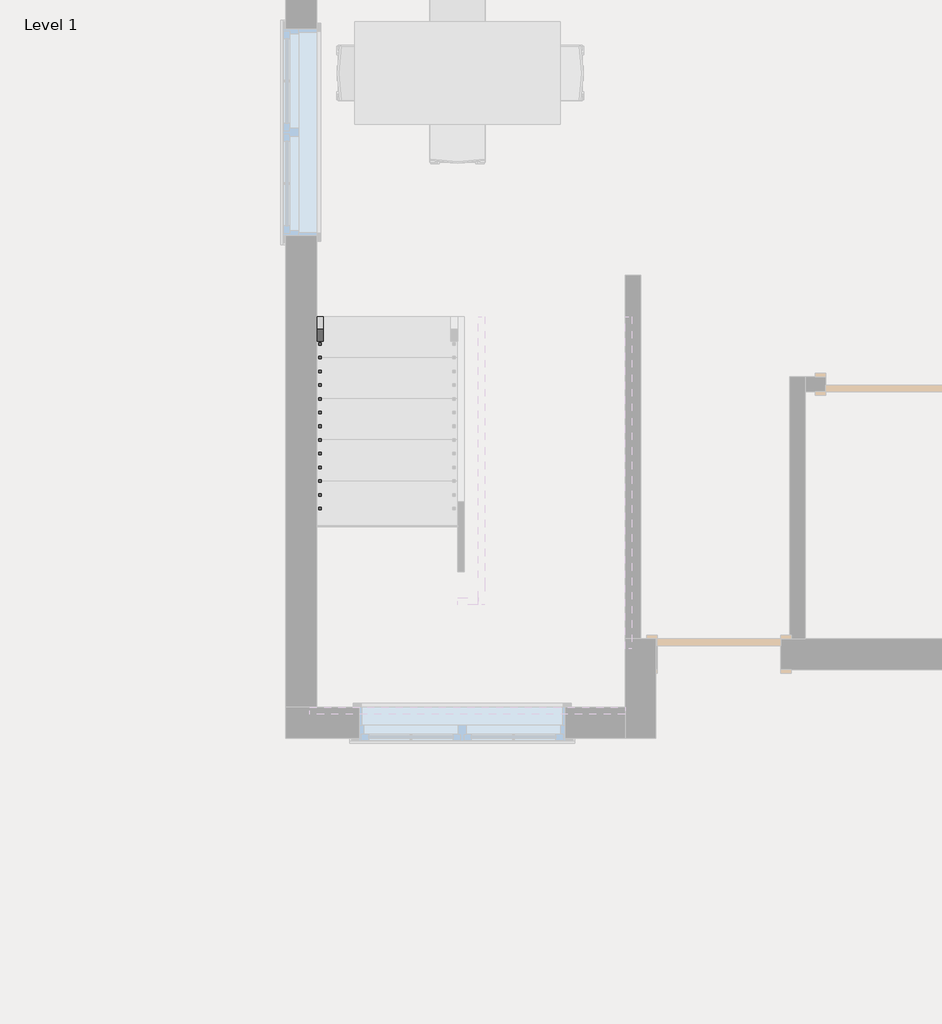
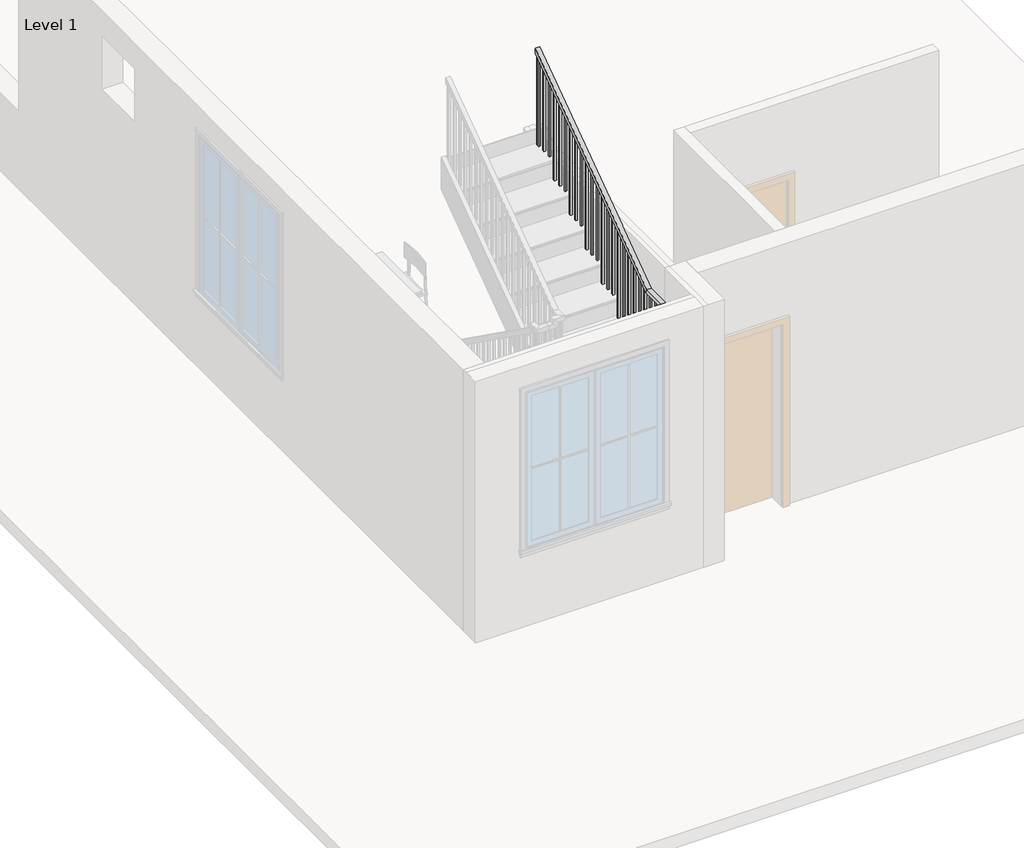
# One storey, part 2 of 3: 1 railing.
"""IFC4 building model written with IfcOpenShell, lengths in millimetres."""

from ifc_helpers import new_model, si_unit, frame, origin, place, context, project, spatial, polyline, outline, extrude, faceted_brep, element, save

model = new_model("IFC4")

# Units and contexts
model_context = context("Model", 3, world=origin())
ifc_project = project(units=[si_unit("LENGTHUNIT", "METRE", prefix="MILLI")], contexts=[model_context])

# Site, building, storey
site = spatial("IfcSite", under=ifc_project)
building = spatial("IfcBuilding", under=site)
storey = spatial("IfcBuildingStorey", under=building, Name="Level 1", Elevation=0.0)

# Railing
placement = place(None, origin())
element("IfcRailing", 1, ObjectType="Handrail - Rectangular", at=placement, inside=storey, context=model_context, shape_type="SolidModel", body=[
    faceted_brep([(-4181.480864, -3571.6080018, 1132.1142857), (-4181.480864, -3571.6080018, 1069.6859823), (-4232.280864, -3571.6080018, 1069.6859823), (-4232.280864, -3571.6080018, 1132.1142857), (-4181.480864, -5705.2080018, 2656.1142857), (-4181.480864, -5721.4876265, 2605.3142857), (-4232.280864, -5721.4876265, 2605.3142857), (-4232.280864, -5705.2080018, 2656.1142857), (-4181.480864, -6416.4080018, 2656.1142857), (-4181.480864, -6416.4080018, 2605.3142857), (-4232.280864, -6467.2080018, 2605.3142857), (-4232.280864, -6467.2080018, 2656.1142857), (-1997.080864, -6416.4080018, 2656.1142857), (-1997.080864, -6416.4080018, 2605.3142857), (-1946.280864, -6467.2080018, 2605.3142857), (-1946.280864, -6467.2080018, 2656.1142857), (-1997.080864, -5705.2080018, 2656.1142857), (-1997.080864, -5688.9283771, 2605.3142857), (-1946.280864, -5688.9283771, 2605.3142857), (-1946.280864, -5705.2080018, 2656.1142857), (-1997.080864, -3571.6080018, 4180.1142857), (-1946.280864, -3571.6080018, 4180.1142857), (-1946.280864, -3571.6080018, 4117.6859823), (-1997.080864, -3571.6080018, 4117.6859823)], [[[0, 1, 2, 3]], [[1, 0, 4, 5]], [[2, 1, 5, 6]], [[3, 2, 6, 7]], [[0, 3, 7, 4]], [[5, 4, 8, 9]], [[6, 5, 9, 10]], [[7, 6, 10, 11]], [[4, 7, 11, 8]], [[9, 8, 12, 13]], [[10, 9, 13, 14]], [[11, 10, 14, 15]], [[8, 11, 15, 12]], [[13, 12, 16, 17]], [[14, 13, 17, 18]], [[15, 14, 18, 19]], [[12, 15, 19, 16]], [[20, 21, 22, 23]], [[17, 16, 20, 23]], [[18, 17, 23, 22]], [[19, 18, 22, 21]], [[16, 19, 21, 20]]]),
    extrude(outline(polyline([(-3606.5330018, 4092.7395538), (-3587.4830018, 4106.3466966), (-3587.4830018, 3048.0), (-3606.5330018, 3048.0), (-3606.5330018, 4092.7395538)])), frame((-1981.205864, 0.0, 0.0), z_axis=(1.0, 0.0, 0.0), x_axis=(0.0, 1.0, 0.0)), (0.0, 0.0, 1.0), 19.05),
    extrude(outline(polyline([(-3708.1330018, 4020.1681252), (-3689.0830018, 4033.7752681), (-3689.0830018, 3048.0), (-3708.1330018, 3048.0), (-3708.1330018, 4020.1681252)])), frame((-1981.205864, 0.0, 0.0), z_axis=(1.0, 0.0, 0.0), x_axis=(0.0, 1.0, 0.0)), (0.0, 0.0, 1.0), 19.05),
    extrude(outline(polyline([(-3809.7330018, 3947.5966966), (-3790.6830018, 3961.2038395), (-3790.6830018, 3048.0), (-3809.7330018, 3048.0), (-3809.7330018, 3947.5966966)])), frame((-1981.205864, 0.0, 0.0), z_axis=(1.0, 0.0, 0.0), x_axis=(0.0, 1.0, 0.0)), (0.0, 0.0, 1.0), 19.05),
    extrude(outline(polyline([(-3911.3330018, 3875.0252681), (-3892.2830018, 3888.6324109), (-3892.2830018, 2830.2857143), (-3911.3330018, 2830.2857143), (-3911.3330018, 3875.0252681)])), frame((-1981.205864, 0.0, 0.0), z_axis=(1.0, 0.0, 0.0), x_axis=(0.0, 1.0, 0.0)), (0.0, 0.0, 1.0), 19.05),
    extrude(outline(polyline([(-4012.9330018, 3802.4538395), (-3993.8830018, 3816.0609823), (-3993.8830018, 2830.2857143), (-4012.9330018, 2830.2857143), (-4012.9330018, 3802.4538395)])), frame((-1981.205864, 0.0, 0.0), z_axis=(1.0, 0.0, 0.0), x_axis=(0.0, 1.0, 0.0)), (0.0, 0.0, 1.0), 19.05),
    extrude(outline(polyline([(-4114.5330018, 3729.8824109), (-4095.4830018, 3743.4895538), (-4095.4830018, 2830.2857143), (-4114.5330018, 2830.2857143), (-4114.5330018, 3729.8824109)])), frame((-1981.205864, 0.0, 0.0), z_axis=(1.0, 0.0, 0.0), x_axis=(0.0, 1.0, 0.0)), (0.0, 0.0, 1.0), 19.05),
    extrude(outline(polyline([(-4216.1330018, 3657.3109823), (-4197.0830018, 3670.9181252), (-4197.0830018, 2612.5714286), (-4216.1330018, 2612.5714286), (-4216.1330018, 3657.3109823)])), frame((-1981.205864, 0.0, 0.0), z_axis=(1.0, 0.0, 0.0), x_axis=(0.0, 1.0, 0.0)), (0.0, 0.0, 1.0), 19.05),
    extrude(outline(polyline([(-4317.7330018, 3584.7395538), (-4298.6830018, 3598.3466966), (-4298.6830018, 2612.5714286), (-4317.7330018, 2612.5714286), (-4317.7330018, 3584.7395538)])), frame((-1981.205864, 0.0, 0.0), z_axis=(1.0, 0.0, 0.0), x_axis=(0.0, 1.0, 0.0)), (0.0, 0.0, 1.0), 19.05),
    extrude(outline(polyline([(-4419.3330018, 3512.1681252), (-4400.2830018, 3525.7752681), (-4400.2830018, 2612.5714286), (-4419.3330018, 2612.5714286), (-4419.3330018, 3512.1681252)])), frame((-1981.205864, 0.0, 0.0), z_axis=(1.0, 0.0, 0.0), x_axis=(0.0, 1.0, 0.0)), (0.0, 0.0, 1.0), 19.05),
    extrude(outline(polyline([(-4520.9330018, 3439.5966966), (-4501.8830018, 3453.2038395), (-4501.8830018, 2394.8571429), (-4520.9330018, 2394.8571429), (-4520.9330018, 3439.5966966)])), frame((-1981.205864, 0.0, 0.0), z_axis=(1.0, 0.0, 0.0), x_axis=(0.0, 1.0, 0.0)), (0.0, 0.0, 1.0), 19.05),
    extrude(outline(polyline([(-4622.5330018, 3367.0252681), (-4603.4830018, 3380.6324109), (-4603.4830018, 2394.8571429), (-4622.5330018, 2394.8571429), (-4622.5330018, 3367.0252681)])), frame((-1981.205864, 0.0, 0.0), z_axis=(1.0, 0.0, 0.0), x_axis=(0.0, 1.0, 0.0)), (0.0, 0.0, 1.0), 19.05),
    extrude(outline(polyline([(-4724.1330018, 3294.4538395), (-4705.0830018, 3308.0609823), (-4705.0830018, 2394.8571429), (-4724.1330018, 2394.8571429), (-4724.1330018, 3294.4538395)])), frame((-1981.205864, 0.0, 0.0), z_axis=(1.0, 0.0, 0.0), x_axis=(0.0, 1.0, 0.0)), (0.0, 0.0, 1.0), 19.05),
    extrude(outline(polyline([(-4825.7330018, 3221.8824109), (-4806.6830018, 3235.4895538), (-4806.6830018, 2177.1428571), (-4825.7330018, 2177.1428571), (-4825.7330018, 3221.8824109)])), frame((-1981.205864, 0.0, 0.0), z_axis=(1.0, 0.0, 0.0), x_axis=(0.0, 1.0, 0.0)), (0.0, 0.0, 1.0), 19.05),
    extrude(outline(polyline([(-4927.3330018, 3149.3109823), (-4908.2830018, 3162.9181252), (-4908.2830018, 2177.1428571), (-4927.3330018, 2177.1428571), (-4927.3330018, 3149.3109823)])), frame((-1981.205864, 0.0, 0.0), z_axis=(1.0, 0.0, 0.0), x_axis=(0.0, 1.0, 0.0)), (0.0, 0.0, 1.0), 19.05),
    extrude(outline(polyline([(-5028.9330018, 3076.7395538), (-5009.8830018, 3090.3466966), (-5009.8830018, 2177.1428571), (-5028.9330018, 2177.1428571), (-5028.9330018, 3076.7395538)])), frame((-1981.205864, 0.0, 0.0), z_axis=(1.0, 0.0, 0.0), x_axis=(0.0, 1.0, 0.0)), (0.0, 0.0, 1.0), 19.05),
    extrude(outline(polyline([(-5130.5330018, 3004.1681252), (-5111.4830018, 3017.7752681), (-5111.4830018, 1959.4285714), (-5130.5330018, 1959.4285714), (-5130.5330018, 3004.1681252)])), frame((-1981.205864, 0.0, 0.0), z_axis=(1.0, 0.0, 0.0), x_axis=(0.0, 1.0, 0.0)), (0.0, 0.0, 1.0), 19.05),
    extrude(outline(polyline([(-5232.1330018, 2931.5966966), (-5213.0830018, 2945.2038395), (-5213.0830018, 1959.4285714), (-5232.1330018, 1959.4285714), (-5232.1330018, 2931.5966966)])), frame((-1981.205864, 0.0, 0.0), z_axis=(1.0, 0.0, 0.0), x_axis=(0.0, 1.0, 0.0)), (0.0, 0.0, 1.0), 19.05),
    extrude(outline(polyline([(-5333.7330018, 2859.0252681), (-5314.6830018, 2872.6324109), (-5314.6830018, 1959.4285714), (-5333.7330018, 1959.4285714), (-5333.7330018, 2859.0252681)])), frame((-1981.205864, 0.0, 0.0), z_axis=(1.0, 0.0, 0.0), x_axis=(0.0, 1.0, 0.0)), (0.0, 0.0, 1.0), 19.05),
    extrude(outline(polyline([(-5435.3330018, 2786.4538395), (-5416.2830018, 2800.0609823), (-5416.2830018, 1741.7142857), (-5435.3330018, 1741.7142857), (-5435.3330018, 2786.4538395)])), frame((-1981.205864, 0.0, 0.0), z_axis=(1.0, 0.0, 0.0), x_axis=(0.0, 1.0, 0.0)), (0.0, 0.0, 1.0), 19.05),
    extrude(outline(polyline([(-5536.9330018, 2713.8824109), (-5517.8830018, 2727.4895538), (-5517.8830018, 1741.7142857), (-5536.9330018, 1741.7142857), (-5536.9330018, 2713.8824109)])), frame((-1981.205864, 0.0, 0.0), z_axis=(1.0, 0.0, 0.0), x_axis=(0.0, 1.0, 0.0)), (0.0, 0.0, 1.0), 19.05),
    extrude(outline(polyline([(-5638.5330018, 2641.3109823), (-5619.4830018, 2654.9181252), (-5619.4830018, 1741.7142857), (-5638.5330018, 1741.7142857), (-5638.5330018, 2641.3109823)])), frame((-1981.205864, 0.0, 0.0), z_axis=(1.0, 0.0, 0.0), x_axis=(0.0, 1.0, 0.0)), (0.0, 0.0, 1.0), 19.05),
    extrude(outline(polyline([(-1962.155864, -5740.1330018), (-1981.205864, -5740.1330018), (-1981.205864, -5721.0830018), (-1962.155864, -5721.0830018), (-1962.155864, -5740.1330018)])), frame((0.0, 0.0, 1741.7142857), z_axis=(0.0, 0.0, 1.0), x_axis=(1.0, 0.0, 0.0)), (0.0, 0.0, 1.0), 863.6),
    extrude(outline(polyline([(-1962.155864, -5841.7330018), (-1981.205864, -5841.7330018), (-1981.205864, -5822.6830018), (-1962.155864, -5822.6830018), (-1962.155864, -5841.7330018)])), frame((0.0, 0.0, 1741.7142857), z_axis=(0.0, 0.0, 1.0), x_axis=(1.0, 0.0, 0.0)), (0.0, 0.0, 1.0), 863.6),
    extrude(outline(polyline([(-1962.155864, -5943.3330018), (-1981.205864, -5943.3330018), (-1981.205864, -5924.2830018), (-1962.155864, -5924.2830018), (-1962.155864, -5943.3330018)])), frame((0.0, 0.0, 1741.7142857), z_axis=(0.0, 0.0, 1.0), x_axis=(1.0, 0.0, 0.0)), (0.0, 0.0, 1.0), 863.6),
    extrude(outline(polyline([(-1962.155864, -6044.9330018), (-1981.205864, -6044.9330018), (-1981.205864, -6025.8830018), (-1962.155864, -6025.8830018), (-1962.155864, -6044.9330018)])), frame((0.0, 0.0, 1741.7142857), z_axis=(0.0, 0.0, 1.0), x_axis=(1.0, 0.0, 0.0)), (0.0, 0.0, 1.0), 863.6),
    extrude(outline(polyline([(-1962.155864, -6146.5330018), (-1981.205864, -6146.5330018), (-1981.205864, -6127.4830018), (-1962.155864, -6127.4830018), (-1962.155864, -6146.5330018)])), frame((0.0, 0.0, 1741.7142857), z_axis=(0.0, 0.0, 1.0), x_axis=(1.0, 0.0, 0.0)), (0.0, 0.0, 1.0), 863.6),
    extrude(outline(polyline([(-1962.155864, -6248.1330018), (-1981.205864, -6248.1330018), (-1981.205864, -6229.0830018), (-1962.155864, -6229.0830018), (-1962.155864, -6248.1330018)])), frame((0.0, 0.0, 1741.7142857), z_axis=(0.0, 0.0, 1.0), x_axis=(1.0, 0.0, 0.0)), (0.0, 0.0, 1.0), 863.6),
    extrude(outline(polyline([(-1962.155864, -6349.7330018), (-1981.205864, -6349.7330018), (-1981.205864, -6330.6830018), (-1962.155864, -6330.6830018), (-1962.155864, -6349.7330018)])), frame((0.0, 0.0, 1741.7142857), z_axis=(0.0, 0.0, 1.0), x_axis=(1.0, 0.0, 0.0)), (0.0, 0.0, 1.0), 863.6),
    extrude(outline(polyline([(-2082.805864, -6451.3330018), (-2082.805864, -6432.2830018), (-2063.755864, -6432.2830018), (-2063.755864, -6451.3330018), (-2082.805864, -6451.3330018)])), frame((0.0, 0.0, 1741.7142857), z_axis=(0.0, 0.0, 1.0), x_axis=(1.0, 0.0, 0.0)), (0.0, 0.0, 1.0), 863.6),
    extrude(outline(polyline([(-2184.405864, -6451.3330018), (-2184.405864, -6432.2830018), (-2165.355864, -6432.2830018), (-2165.355864, -6451.3330018), (-2184.405864, -6451.3330018)])), frame((0.0, 0.0, 1741.7142857), z_axis=(0.0, 0.0, 1.0), x_axis=(1.0, 0.0, 0.0)), (0.0, 0.0, 1.0), 863.6),
    extrude(outline(polyline([(-2286.005864, -6451.3330018), (-2286.005864, -6432.2830018), (-2266.955864, -6432.2830018), (-2266.955864, -6451.3330018), (-2286.005864, -6451.3330018)])), frame((0.0, 0.0, 1741.7142857), z_axis=(0.0, 0.0, 1.0), x_axis=(1.0, 0.0, 0.0)), (0.0, 0.0, 1.0), 863.6),
    extrude(outline(polyline([(-2387.605864, -6451.3330018), (-2387.605864, -6432.2830018), (-2368.555864, -6432.2830018), (-2368.555864, -6451.3330018), (-2387.605864, -6451.3330018)])), frame((0.0, 0.0, 1741.7142857), z_axis=(0.0, 0.0, 1.0), x_axis=(1.0, 0.0, 0.0)), (0.0, 0.0, 1.0), 863.6),
    extrude(outline(polyline([(-2489.205864, -6451.3330018), (-2489.205864, -6432.2830018), (-2470.155864, -6432.2830018), (-2470.155864, -6451.3330018), (-2489.205864, -6451.3330018)])), frame((0.0, 0.0, 1741.7142857), z_axis=(0.0, 0.0, 1.0), x_axis=(1.0, 0.0, 0.0)), (0.0, 0.0, 1.0), 863.6),
    extrude(outline(polyline([(-2590.805864, -6451.3330018), (-2590.805864, -6432.2830018), (-2571.755864, -6432.2830018), (-2571.755864, -6451.3330018), (-2590.805864, -6451.3330018)])), frame((0.0, 0.0, 1741.7142857), z_axis=(0.0, 0.0, 1.0), x_axis=(1.0, 0.0, 0.0)), (0.0, 0.0, 1.0), 863.6),
    extrude(outline(polyline([(-2692.405864, -6451.3330018), (-2692.405864, -6432.2830018), (-2673.355864, -6432.2830018), (-2673.355864, -6451.3330018), (-2692.405864, -6451.3330018)])), frame((0.0, 0.0, 1741.7142857), z_axis=(0.0, 0.0, 1.0), x_axis=(1.0, 0.0, 0.0)), (0.0, 0.0, 1.0), 863.6),
    extrude(outline(polyline([(-2794.005864, -6451.3330018), (-2794.005864, -6432.2830018), (-2774.955864, -6432.2830018), (-2774.955864, -6451.3330018), (-2794.005864, -6451.3330018)])), frame((0.0, 0.0, 1741.7142857), z_axis=(0.0, 0.0, 1.0), x_axis=(1.0, 0.0, 0.0)), (0.0, 0.0, 1.0), 863.6),
    extrude(outline(polyline([(-2895.605864, -6451.3330018), (-2895.605864, -6432.2830018), (-2876.555864, -6432.2830018), (-2876.555864, -6451.3330018), (-2895.605864, -6451.3330018)])), frame((0.0, 0.0, 1741.7142857), z_axis=(0.0, 0.0, 1.0), x_axis=(1.0, 0.0, 0.0)), (0.0, 0.0, 1.0), 863.6),
    extrude(outline(polyline([(-2997.205864, -6451.3330018), (-2997.205864, -6432.2830018), (-2978.155864, -6432.2830018), (-2978.155864, -6451.3330018), (-2997.205864, -6451.3330018)])), frame((0.0, 0.0, 1741.7142857), z_axis=(0.0, 0.0, 1.0), x_axis=(1.0, 0.0, 0.0)), (0.0, 0.0, 1.0), 863.6),
    extrude(outline(polyline([(-3098.805864, -6451.3330018), (-3098.805864, -6432.2830018), (-3079.755864, -6432.2830018), (-3079.755864, -6451.3330018), (-3098.805864, -6451.3330018)])), frame((0.0, 0.0, 1741.7142857), z_axis=(0.0, 0.0, 1.0), x_axis=(1.0, 0.0, 0.0)), (0.0, 0.0, 1.0), 863.6),
    extrude(outline(polyline([(-3200.405864, -6451.3330018), (-3200.405864, -6432.2830018), (-3181.355864, -6432.2830018), (-3181.355864, -6451.3330018), (-3200.405864, -6451.3330018)])), frame((0.0, 0.0, 1741.7142857), z_axis=(0.0, 0.0, 1.0), x_axis=(1.0, 0.0, 0.0)), (0.0, 0.0, 1.0), 863.6),
    extrude(outline(polyline([(-3302.005864, -6451.3330018), (-3302.005864, -6432.2830018), (-3282.955864, -6432.2830018), (-3282.955864, -6451.3330018), (-3302.005864, -6451.3330018)])), frame((0.0, 0.0, 1741.7142857), z_axis=(0.0, 0.0, 1.0), x_axis=(1.0, 0.0, 0.0)), (0.0, 0.0, 1.0), 863.6),
    extrude(outline(polyline([(-3403.605864, -6451.3330018), (-3403.605864, -6432.2830018), (-3384.555864, -6432.2830018), (-3384.555864, -6451.3330018), (-3403.605864, -6451.3330018)])), frame((0.0, 0.0, 1741.7142857), z_axis=(0.0, 0.0, 1.0), x_axis=(1.0, 0.0, 0.0)), (0.0, 0.0, 1.0), 863.6),
    extrude(outline(polyline([(-3505.205864, -6451.3330018), (-3505.205864, -6432.2830018), (-3486.155864, -6432.2830018), (-3486.155864, -6451.3330018), (-3505.205864, -6451.3330018)])), frame((0.0, 0.0, 1741.7142857), z_axis=(0.0, 0.0, 1.0), x_axis=(1.0, 0.0, 0.0)), (0.0, 0.0, 1.0), 863.6),
    extrude(outline(polyline([(-3606.805864, -6451.3330018), (-3606.805864, -6432.2830018), (-3587.755864, -6432.2830018), (-3587.755864, -6451.3330018), (-3606.805864, -6451.3330018)])), frame((0.0, 0.0, 1741.7142857), z_axis=(0.0, 0.0, 1.0), x_axis=(1.0, 0.0, 0.0)), (0.0, 0.0, 1.0), 863.6),
    extrude(outline(polyline([(-3708.405864, -6451.3330018), (-3708.405864, -6432.2830018), (-3689.355864, -6432.2830018), (-3689.355864, -6451.3330018), (-3708.405864, -6451.3330018)])), frame((0.0, 0.0, 1741.7142857), z_axis=(0.0, 0.0, 1.0), x_axis=(1.0, 0.0, 0.0)), (0.0, 0.0, 1.0), 863.6),
    extrude(outline(polyline([(-3810.005864, -6451.3330018), (-3810.005864, -6432.2830018), (-3790.955864, -6432.2830018), (-3790.955864, -6451.3330018), (-3810.005864, -6451.3330018)])), frame((0.0, 0.0, 1741.7142857), z_axis=(0.0, 0.0, 1.0), x_axis=(1.0, 0.0, 0.0)), (0.0, 0.0, 1.0), 863.6),
    extrude(outline(polyline([(-3911.605864, -6451.3330018), (-3911.605864, -6432.2830018), (-3892.555864, -6432.2830018), (-3892.555864, -6451.3330018), (-3911.605864, -6451.3330018)])), frame((0.0, 0.0, 1741.7142857), z_axis=(0.0, 0.0, 1.0), x_axis=(1.0, 0.0, 0.0)), (0.0, 0.0, 1.0), 863.6),
    extrude(outline(polyline([(-4013.205864, -6451.3330018), (-4013.205864, -6432.2830018), (-3994.155864, -6432.2830018), (-3994.155864, -6451.3330018), (-4013.205864, -6451.3330018)])), frame((0.0, 0.0, 1741.7142857), z_axis=(0.0, 0.0, 1.0), x_axis=(1.0, 0.0, 0.0)), (0.0, 0.0, 1.0), 863.6),
    extrude(outline(polyline([(-4114.805864, -6451.3330018), (-4114.805864, -6432.2830018), (-4095.755864, -6432.2830018), (-4095.755864, -6451.3330018), (-4114.805864, -6451.3330018)])), frame((0.0, 0.0, 1741.7142857), z_axis=(0.0, 0.0, 1.0), x_axis=(1.0, 0.0, 0.0)), (0.0, 0.0, 1.0), 863.6),
    extrude(outline(polyline([(-4216.405864, -6406.8830018), (-4197.355864, -6406.8830018), (-4197.355864, -6425.9330018), (-4216.405864, -6425.9330018), (-4216.405864, -6406.8830018)])), frame((0.0, 0.0, 1741.7142857), z_axis=(0.0, 0.0, 1.0), x_axis=(1.0, 0.0, 0.0)), (0.0, 0.0, 1.0), 863.6),
    extrude(outline(polyline([(-4216.405864, -6305.2830018), (-4197.355864, -6305.2830018), (-4197.355864, -6324.3330018), (-4216.405864, -6324.3330018), (-4216.405864, -6305.2830018)])), frame((0.0, 0.0, 1741.7142857), z_axis=(0.0, 0.0, 1.0), x_axis=(1.0, 0.0, 0.0)), (0.0, 0.0, 1.0), 863.6),
    extrude(outline(polyline([(-4216.405864, -6203.6830018), (-4197.355864, -6203.6830018), (-4197.355864, -6222.7330018), (-4216.405864, -6222.7330018), (-4216.405864, -6203.6830018)])), frame((0.0, 0.0, 1741.7142857), z_axis=(0.0, 0.0, 1.0), x_axis=(1.0, 0.0, 0.0)), (0.0, 0.0, 1.0), 863.6),
    extrude(outline(polyline([(-4216.405864, -6102.0830018), (-4197.355864, -6102.0830018), (-4197.355864, -6121.1330018), (-4216.405864, -6121.1330018), (-4216.405864, -6102.0830018)])), frame((0.0, 0.0, 1741.7142857), z_axis=(0.0, 0.0, 1.0), x_axis=(1.0, 0.0, 0.0)), (0.0, 0.0, 1.0), 863.6),
    extrude(outline(polyline([(-4216.405864, -6000.4830018), (-4197.355864, -6000.4830018), (-4197.355864, -6019.5330018), (-4216.405864, -6019.5330018), (-4216.405864, -6000.4830018)])), frame((0.0, 0.0, 1741.7142857), z_axis=(0.0, 0.0, 1.0), x_axis=(1.0, 0.0, 0.0)), (0.0, 0.0, 1.0), 863.6),
    extrude(outline(polyline([(-4216.405864, -5898.8830018), (-4197.355864, -5898.8830018), (-4197.355864, -5917.9330018), (-4216.405864, -5917.9330018), (-4216.405864, -5898.8830018)])), frame((0.0, 0.0, 1741.7142857), z_axis=(0.0, 0.0, 1.0), x_axis=(1.0, 0.0, 0.0)), (0.0, 0.0, 1.0), 863.6),
    extrude(outline(polyline([(-4216.405864, -5797.2830018), (-4197.355864, -5797.2830018), (-4197.355864, -5816.3330018), (-4216.405864, -5816.3330018), (-4216.405864, -5797.2830018)])), frame((0.0, 0.0, 1741.7142857), z_axis=(0.0, 0.0, 1.0), x_axis=(1.0, 0.0, 0.0)), (0.0, 0.0, 1.0), 863.6),
    extrude(outline(polyline([(-5714.7330018, 2600.4895538), (-5695.6830018, 2586.8824109), (-5695.6830018, 1741.7142857), (-5714.7330018, 1741.7142857), (-5714.7330018, 2600.4895538)])), frame((-4216.405864, 0.0, 0.0), z_axis=(1.0, 0.0, 0.0), x_axis=(0.0, 1.0, 0.0)), (0.0, 0.0, 1.0), 19.05),
    extrude(outline(polyline([(-5613.1330018, 2527.9181252), (-5594.0830018, 2514.3109823), (-5594.0830018, 1524.0), (-5613.1330018, 1524.0), (-5613.1330018, 2527.9181252)])), frame((-4216.405864, 0.0, 0.0), z_axis=(1.0, 0.0, 0.0), x_axis=(0.0, 1.0, 0.0)), (0.0, 0.0, 1.0), 19.05),
    extrude(outline(polyline([(-5511.5330018, 2455.3466966), (-5492.4830018, 2441.7395538), (-5492.4830018, 1524.0), (-5511.5330018, 1524.0), (-5511.5330018, 2455.3466966)])), frame((-4216.405864, 0.0, 0.0), z_axis=(1.0, 0.0, 0.0), x_axis=(0.0, 1.0, 0.0)), (0.0, 0.0, 1.0), 19.05),
    extrude(outline(polyline([(-5409.9330018, 2382.7752681), (-5390.8830018, 2369.1681252), (-5390.8830018, 1524.0), (-5409.9330018, 1524.0), (-5409.9330018, 2382.7752681)])), frame((-4216.405864, 0.0, 0.0), z_axis=(1.0, 0.0, 0.0), x_axis=(0.0, 1.0, 0.0)), (0.0, 0.0, 1.0), 19.05),
    extrude(outline(polyline([(-5308.3330018, 2310.2038395), (-5289.2830018, 2296.5966966), (-5289.2830018, 1306.2857143), (-5308.3330018, 1306.2857143), (-5308.3330018, 2310.2038395)])), frame((-4216.405864, 0.0, 0.0), z_axis=(1.0, 0.0, 0.0), x_axis=(0.0, 1.0, 0.0)), (0.0, 0.0, 1.0), 19.05),
    extrude(outline(polyline([(-5206.7330018, 2237.6324109), (-5187.6830018, 2224.0252681), (-5187.6830018, 1306.2857143), (-5206.7330018, 1306.2857143), (-5206.7330018, 2237.6324109)])), frame((-4216.405864, 0.0, 0.0), z_axis=(1.0, 0.0, 0.0), x_axis=(0.0, 1.0, 0.0)), (0.0, 0.0, 1.0), 19.05),
    extrude(outline(polyline([(-5105.1330018, 2165.0609823), (-5086.0830018, 2151.4538395), (-5086.0830018, 1306.2857143), (-5105.1330018, 1306.2857143), (-5105.1330018, 2165.0609823)])), frame((-4216.405864, 0.0, 0.0), z_axis=(1.0, 0.0, 0.0), x_axis=(0.0, 1.0, 0.0)), (0.0, 0.0, 1.0), 19.05),
    extrude(outline(polyline([(-5003.5330018, 2092.4895538), (-4984.4830018, 2078.8824109), (-4984.4830018, 1088.5714286), (-5003.5330018, 1088.5714286), (-5003.5330018, 2092.4895538)])), frame((-4216.405864, 0.0, 0.0), z_axis=(1.0, 0.0, 0.0), x_axis=(0.0, 1.0, 0.0)), (0.0, 0.0, 1.0), 19.05),
    extrude(outline(polyline([(-4901.9330018, 2019.9181252), (-4882.8830018, 2006.3109823), (-4882.8830018, 1088.5714286), (-4901.9330018, 1088.5714286), (-4901.9330018, 2019.9181252)])), frame((-4216.405864, 0.0, 0.0), z_axis=(1.0, 0.0, 0.0), x_axis=(0.0, 1.0, 0.0)), (0.0, 0.0, 1.0), 19.05),
    extrude(outline(polyline([(-4800.3330018, 1947.3466966), (-4781.2830018, 1933.7395538), (-4781.2830018, 1088.5714286), (-4800.3330018, 1088.5714286), (-4800.3330018, 1947.3466966)])), frame((-4216.405864, 0.0, 0.0), z_axis=(1.0, 0.0, 0.0), x_axis=(0.0, 1.0, 0.0)), (0.0, 0.0, 1.0), 19.05),
    extrude(outline(polyline([(-4698.7330018, 1874.7752681), (-4679.6830018, 1861.1681252), (-4679.6830018, 870.8571429), (-4698.7330018, 870.8571429), (-4698.7330018, 1874.7752681)])), frame((-4216.405864, 0.0, 0.0), z_axis=(1.0, 0.0, 0.0), x_axis=(0.0, 1.0, 0.0)), (0.0, 0.0, 1.0), 19.05),
    extrude(outline(polyline([(-4597.1330018, 1802.2038395), (-4578.0830018, 1788.5966966), (-4578.0830018, 870.8571429), (-4597.1330018, 870.8571429), (-4597.1330018, 1802.2038395)])), frame((-4216.405864, 0.0, 0.0), z_axis=(1.0, 0.0, 0.0), x_axis=(0.0, 1.0, 0.0)), (0.0, 0.0, 1.0), 19.05),
    extrude(outline(polyline([(-4495.5330018, 1729.6324109), (-4476.4830018, 1716.0252681), (-4476.4830018, 870.8571429), (-4495.5330018, 870.8571429), (-4495.5330018, 1729.6324109)])), frame((-4216.405864, 0.0, 0.0), z_axis=(1.0, 0.0, 0.0), x_axis=(0.0, 1.0, 0.0)), (0.0, 0.0, 1.0), 19.05),
    extrude(outline(polyline([(-4393.9330018, 1657.0609823), (-4374.8830018, 1643.4538395), (-4374.8830018, 653.1428571), (-4393.9330018, 653.1428571), (-4393.9330018, 1657.0609823)])), frame((-4216.405864, 0.0, 0.0), z_axis=(1.0, 0.0, 0.0), x_axis=(0.0, 1.0, 0.0)), (0.0, 0.0, 1.0), 19.05),
    extrude(outline(polyline([(-4292.3330018, 1584.4895538), (-4273.2830018, 1570.8824109), (-4273.2830018, 653.1428571), (-4292.3330018, 653.1428571), (-4292.3330018, 1584.4895538)])), frame((-4216.405864, 0.0, 0.0), z_axis=(1.0, 0.0, 0.0), x_axis=(0.0, 1.0, 0.0)), (0.0, 0.0, 1.0), 19.05),
    extrude(outline(polyline([(-4190.7330018, 1511.9181252), (-4171.6830018, 1498.3109823), (-4171.6830018, 653.1428571), (-4190.7330018, 653.1428571), (-4190.7330018, 1511.9181252)])), frame((-4216.405864, 0.0, 0.0), z_axis=(1.0, 0.0, 0.0), x_axis=(0.0, 1.0, 0.0)), (0.0, 0.0, 1.0), 19.05),
    extrude(outline(polyline([(-4089.1330018, 1439.3466966), (-4070.0830018, 1425.7395538), (-4070.0830018, 435.4285714), (-4089.1330018, 435.4285714), (-4089.1330018, 1439.3466966)])), frame((-4216.405864, 0.0, 0.0), z_axis=(1.0, 0.0, 0.0), x_axis=(0.0, 1.0, 0.0)), (0.0, 0.0, 1.0), 19.05),
    extrude(outline(polyline([(-3987.5330018, 1366.7752681), (-3968.4830018, 1353.1681252), (-3968.4830018, 435.4285714), (-3987.5330018, 435.4285714), (-3987.5330018, 1366.7752681)])), frame((-4216.405864, 0.0, 0.0), z_axis=(1.0, 0.0, 0.0), x_axis=(0.0, 1.0, 0.0)), (0.0, 0.0, 1.0), 19.05),
    extrude(outline(polyline([(-3885.9330018, 1294.2038395), (-3866.8830018, 1280.5966966), (-3866.8830018, 435.4285714), (-3885.9330018, 435.4285714), (-3885.9330018, 1294.2038395)])), frame((-4216.405864, 0.0, 0.0), z_axis=(1.0, 0.0, 0.0), x_axis=(0.0, 1.0, 0.0)), (0.0, 0.0, 1.0), 19.05),
    extrude(outline(polyline([(-3784.3330018, 1221.6324109), (-3765.2830018, 1208.0252681), (-3765.2830018, 217.7142857), (-3784.3330018, 217.7142857), (-3784.3330018, 1221.6324109)])), frame((-4216.405864, 0.0, 0.0), z_axis=(1.0, 0.0, 0.0), x_axis=(0.0, 1.0, 0.0)), (0.0, 0.0, 1.0), 19.05),
    extrude(outline(polyline([(-3682.7330018, 1149.0609823), (-3663.6830018, 1135.4538395), (-3663.6830018, 217.7142857), (-3682.7330018, 217.7142857), (-3682.7330018, 1149.0609823)])), frame((-4216.405864, 0.0, 0.0), z_axis=(1.0, 0.0, 0.0), x_axis=(0.0, 1.0, 0.0)), (0.0, 0.0, 1.0), 19.05),
    extrude(outline(polyline([(-1981.205864, -6451.3330018), (-1981.205864, -6432.2830018), (-1962.155864, -6432.2830018), (-1962.155864, -6451.3330018), (-1981.205864, -6451.3330018)])), frame((0.0, 0.0, 1741.7142857), z_axis=(0.0, 0.0, 1.0), x_axis=(1.0, 0.0, 0.0)), (0.0, 0.0, 1.0), 863.6),
    extrude(outline(polyline([(-4216.405864, -6432.2830018), (-4197.355864, -6432.2830018), (-4197.355864, -6451.3330018), (-4216.405864, -6451.3330018), (-4216.405864, -6432.2830018)])), frame((0.0, 0.0, 1741.7142857), z_axis=(0.0, 0.0, 1.0), x_axis=(1.0, 0.0, 0.0)), (0.0, 0.0, 1.0), 863.6),
    extrude(outline(polyline([(-3590.6580018, 4104.0788395), (-3571.6080018, 4117.6859823), (-3571.6080018, 3048.0), (-3590.6580018, 3048.0), (-3590.6580018, 4104.0788395)])), frame((-1981.205864, 0.0, 0.0), z_axis=(1.0, 0.0, 0.0), x_axis=(0.0, 1.0, 0.0)), (0.0, 0.0, 1.0), 19.05),
    extrude(outline(polyline([(-3590.6580018, 1083.2931252), (-3571.6080018, 1069.6859823), (-3571.6080018, 217.7142857), (-3590.6580018, 217.7142857), (-3590.6580018, 1083.2931252)])), frame((-4216.405864, 0.0, 0.0), z_axis=(1.0, 0.0, 0.0), x_axis=(0.0, 1.0, 0.0)), (0.0, 0.0, 1.0), 19.05),
])

save(model, "model.ifc")

# Revit data of these elements
# Type "Handrail - Rectangular"
#   Assembly Code = "C2010400"
#   built-in parameter 1008612 = 0.0416667 (stored number, unit not read)
#   built-in parameter 1008611 = 0.0416667 (stored number, unit not read)
#   built-in parameter 1008609 = 0.333333 (stored number, unit not read)
#   built-in parameter 1008604 = 0.166667 (stored number, unit not read)
#   built-in parameter 1008603 = 0.166667 (stored number, unit not read)
#   Railing Height = 3' - 0"
#   built-in parameter 1008630 = 2
#   built-in parameter 1008610 = 2
#   built-in parameter 1008618 = Baluster - Square : 3/4"
# Element 1 (IfcRailing, "Handrail - Rectangular")
#   Phase Created = New Construction
